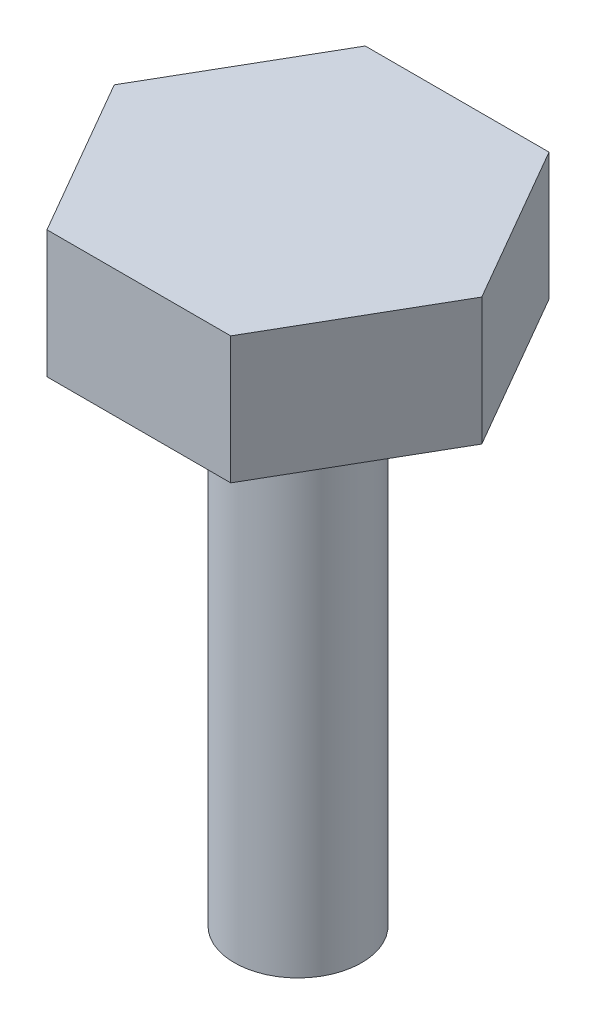
SolidWorks part; units mm, degrees
material "Plain Carbon Steel"
ref_plane "Front Plane" through (0, 0, 0) normal (0, 0, 1) x (1, 0, 0)
ref_plane "Top Plane" through (0, 0, 0) normal (0, 1, 0) x (1, 0, 0)
ref_plane "Right Plane" through (0, 0, 0) normal (1, 0, 0) x (0, 0, -1)
sketch "Hex Head Sketch 50AF" plane through (0, 0, 0) normal (0, 1, 0) x (1, 0, 0)
  line L1 (28.8675, 0) -> (14.4338, 25)
  line L2 (14.4338, 25) -> (-14.4338, 25)
  line L3 (-14.4338, 25) -> (-28.8675, 0)
  line L4 (-28.8675, 0) -> (-14.4338, -25)
  line L5 (-14.4338, -25) -> (14.4338, -25)
  line L6 (14.4338, -25) -> (28.8675, 0)
  circle A0 centre (0, 0) radius 25 construction
  dimension "50" = 50
extrude "Hex Head 50AF x20" add sketch "Hex Head Sketch 50AF" along normal blind 20
sketch "Shank Sketch Ø20" plane through (0, 0, 0) normal (0, -1, 0) x (1, 0, 0)
  circle A0 centre (0, 0) radius 10
  dimension "D1" = 20
extrude "Shank Ø20x80" add sketch "Shank Sketch Ø20" along normal blind 80
